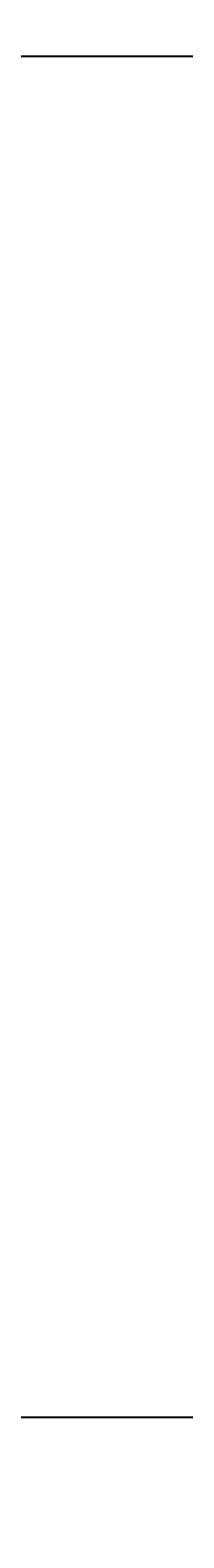
# Model space of a CAD drawing. Units: inches. Extents: x 35362 to 73946, y 43607 to 67532.
# Tile 45 of 134: x 48389 to 48437, y 46091 to 46564. Entities that reach past the tile are written whole.
import ezdxf

# ---------------------------------------------------------------- set-up
doc = ezdxf.new("R2010")
doc.units = ezdxf.units.IN
doc.header["$MEASUREMENT"] = 0
doc.layers.add('A-ANNO-DIMS', color=2, linetype='Continuous', lineweight=18)
doc.styles.get("Standard").update_dxf_attribs({"font": 'arial.ttf'})
doc.dimstyles.get("Standard").update_dxf_attribs({"dimtxt": 0.18, "dimasz": 0.18, "dimexe": 0.18, "dimexo": 0.0625, "dimgap": 0.09, "dimtad": 0, "dimtih": 1, "dimtoh": 1, "dimdec": 4, "dimzin": 0, "dimdsep": 46, "dimtxsty": 'Standard', "dimcen": 0.09, "dimadec": 0, "dimazin": 0, "dimtfac": 1, "dimtdec": 4, "dimtofl": 0, "dimtmove": 0, "dimatfit": 3, "dimfxl": 1, "dimtolj": 1, "dimtzin": 0, "dimarcsym": 0})

# ---------------------------------------------------------------- blocks, each defined once
blk = doc.blocks.new('*D5')
at = {"layer": 'A-ANNO-DIMS', "color": 0, "lineweight": -2, "transparency": 16777216}
for p, q in [((37121.95, 46919.32), (37121.95, 43606.68)), ((69871.5, 45449.83), (69871.5, 43606.68)), ((37122.13, 43606.86), (53496.29, 43606.86)), ((69871.32, 43606.86), (53497.15, 43606.86))]:
    blk.add_line(p, q, dxfattribs=at)
at = {"layer": 'A-ANNO-DIMS', "color": 0, "transparency": 16777216}
for points in [[(37122.13, 43606.89), (37122.13, 43606.83), (37121.95, 43606.86)], [(69871.32, 43606.89), (69871.32, 43606.83), (69871.5, 43606.86)]]:
    blk.add_solid(points, dxfattribs=at)
at = {"layer": 'Defpoints', "color": 0, "transparency": 16777216}
for p in [(37121.95, 46919.38), (69871.5, 45449.89), (69871.5, 43606.86)]:
    blk.add_point(p, dxfattribs=at)
at = {"layer": 'A-ANNO-DIMS', "color": 0, "transparency": 16777216, "insert": (53496.72, 43606.86), "char_height": 0.18, "attachment_point": 5}
blk.add_mtext('\\A1;32750', dxfattribs=at)
blk = doc.blocks.new('*D11')
at = {"layer": 'A-ANNO-DIMS', "color": 0, "lineweight": -2, "transparency": 16777216}
for p, q in [((47978.66, 56028.77), (47978.66, 43606.68)), ((53109.76, 56028.77), (53109.76, 43606.68)), ((47978.84, 43606.86), (50543.87, 43606.86)), ((53109.58, 43606.86), (50544.55, 43606.86))]:
    blk.add_line(p, q, dxfattribs=at)
at = {"layer": 'A-ANNO-DIMS', "color": 0, "transparency": 16777216}
for points in [[(47978.84, 43606.89), (47978.84, 43606.83), (47978.66, 43606.86)], [(53109.58, 43606.89), (53109.58, 43606.83), (53109.76, 43606.86)]]:
    blk.add_solid(points, dxfattribs=at)
at = {"layer": 'Defpoints', "color": 0, "transparency": 16777216}
for p in [(47978.66, 56028.84), (53109.76, 56028.84), (53109.76, 43606.86)]:
    blk.add_point(p, dxfattribs=at)
at = {"layer": 'A-ANNO-DIMS', "color": 0, "transparency": 16777216, "insert": (50544.21, 43606.86), "char_height": 0.18, "attachment_point": 5}
blk.add_mtext('\\A1;5131', dxfattribs=at)
blk = doc.blocks.new('*D13')
at = {"layer": 'A-ANNO-DIMS', "color": 0, "lineweight": -2, "transparency": 16777216}
for p, q in [((48373.49, 51694.02), (48373.49, 43606.68)), ((51029.04, 51694.02), (51029.04, 43606.68)), ((48373.67, 43606.86), (49700.8, 43606.86)), ((51028.86, 43606.86), (49701.73, 43606.86))]:
    blk.add_line(p, q, dxfattribs=at)
at = {"layer": 'A-ANNO-DIMS', "color": 0, "transparency": 16777216}
for points in [[(48373.67, 43606.89), (48373.67, 43606.83), (48373.49, 43606.86)], [(51028.86, 43606.89), (51028.86, 43606.83), (51029.04, 43606.86)]]:
    blk.add_solid(points, dxfattribs=at)
at = {"layer": 'Defpoints', "color": 0, "transparency": 16777216}
for p in [(48373.49, 51694.09), (51029.04, 51694.09), (51029.04, 43606.86)]:
    blk.add_point(p, dxfattribs=at)
at = {"layer": 'A-ANNO-DIMS', "color": 0, "transparency": 16777216, "insert": (49701.27, 43606.86), "char_height": 0.18, "attachment_point": 5}
blk.add_mtext('\\A1;2655.6', dxfattribs=at)
blk = doc.blocks.new('*D67')
at = {"layer": 'A-ANNO-DIMS', "color": 0, "lineweight": -2, "transparency": 16777216}
for p, q in [((56873.54, 53351.53), (35361.77, 53351.53)), ((35361.95, 53351.35), (35361.95, 49400.89)), ((35361.95, 45450.07), (35361.95, 49400.53)), ((53793.58, 45449.89), (35361.77, 45449.89))]:
    blk.add_line(p, q, dxfattribs=at)
at = {"layer": 'A-ANNO-DIMS', "color": 0, "transparency": 16777216}
for points in [[(35361.92, 53351.35), (35361.98, 53351.35), (35361.95, 53351.53)], [(35361.92, 45450.07), (35361.98, 45450.07), (35361.95, 45449.89)]]:
    blk.add_solid(points, dxfattribs=at)
at = {"layer": 'Defpoints', "color": 0, "transparency": 16777216}
for p in [(35361.95, 53351.53), (56873.6, 53351.53), (53793.64, 45449.89)]:
    blk.add_point(p, dxfattribs=at)
at = {"layer": 'A-ANNO-DIMS', "color": 0, "transparency": 16777216, "insert": (35361.95, 49400.71), "char_height": 0.18, "attachment_point": 5}
blk.add_mtext('\\A1;7901.6', dxfattribs=at)
blk = doc.blocks.new('*D76')
at = {"layer": 'A-ANNO-DIMS', "color": 0, "lineweight": -2, "transparency": 16777216}
for p, q in [((54052.84, 46555.29), (35361.77, 46555.29)), ((35361.95, 46555.11), (35361.95, 46342.27)), ((35361.95, 46129.06), (35361.95, 46341.9)), ((53793.58, 46128.88), (35361.77, 46128.88))]:
    blk.add_line(p, q, dxfattribs=at)
at = {"layer": 'A-ANNO-DIMS', "color": 0, "transparency": 16777216}
for points in [[(35361.92, 46555.11), (35361.98, 46555.11), (35361.95, 46555.29)], [(35361.92, 46129.06), (35361.98, 46129.06), (35361.95, 46128.88)]]:
    blk.add_solid(points, dxfattribs=at)
at = {"layer": 'Defpoints', "color": 0, "transparency": 16777216}
for p in [(35361.95, 46555.29), (54052.9, 46555.29), (53793.64, 46128.88)]:
    blk.add_point(p, dxfattribs=at)
at = {"layer": 'A-ANNO-DIMS', "color": 0, "transparency": 16777216, "insert": (35361.95, 46342.09), "char_height": 0.18, "attachment_point": 5}
blk.add_mtext('\\A1;426.4', dxfattribs=at)
blk = doc.blocks.new('*D90')
at = {"layer": 'A-ANNO-DIMS', "color": 0, "lineweight": -2, "transparency": 16777216}
for p, q in [((53707.72, 47291.29), (35361.77, 47291.29)), ((35361.95, 47291.11), (35361.95, 46710.26)), ((35361.95, 46129.06), (35361.95, 46709.9)), ((53793.58, 46128.88), (35361.77, 46128.88))]:
    blk.add_line(p, q, dxfattribs=at)
at = {"layer": 'A-ANNO-DIMS', "color": 0, "transparency": 16777216}
for points in [[(35361.92, 47291.11), (35361.98, 47291.11), (35361.95, 47291.29)], [(35361.92, 46129.06), (35361.98, 46129.06), (35361.95, 46128.88)]]:
    blk.add_solid(points, dxfattribs=at)
at = {"layer": 'Defpoints', "color": 0, "transparency": 16777216}
for p in [(53707.78, 47291.29), (35361.95, 46128.88), (53793.64, 46128.88)]:
    blk.add_point(p, dxfattribs=at)
at = {"layer": 'A-ANNO-DIMS', "color": 0, "transparency": 16777216, "insert": (35361.95, 46710.08), "char_height": 0.18, "attachment_point": 5}
blk.add_mtext('\\A1;1162.4', dxfattribs=at)

msp = doc.modelspace()

# ---------------------------------------------------------------- dimensions: what is measured, and where the dimension line sits
at = {"layer": 'A-ANNO-DIMS'}
for base, p1, p2, override, picture, middle in [((53109.76, 43606.859), (47978.665, 56028.836), (53109.76, 56028.836), {"dimdec": 0, "dimlfac": 1, "dimrnd": 0, "dimzin": 0, "dimdsep": 46, "dimlunit": 2}, '*D11', (50544.212, 43606.859)), ((51029.043, 43606.859), (48373.492, 51694.087), (51029.043, 51694.087), {"dimdec": 1, "dimlfac": 1, "dimrnd": 0, "dimzin": 0, "dimdsep": 46, "dimlunit": 2}, '*D13', (49701.267, 43606.859)), ((69871.496, 43606.859), (37121.949, 46919.381), (69871.496, 45449.894), {"dimdec": 0, "dimlfac": 1, "dimrnd": 0, "dimzin": 0, "dimdsep": 46, "dimlunit": 2}, '*D5', (53496.723, 43606.859))]:
    dim = msp.add_linear_dim(base=base, p1=p1, p2=p2, dimstyle='Standard', override=override, dxfattribs=at)
    dim.commit()
    dim.dimension.update_dxf_attribs({"geometry": picture, "text_midpoint": middle})
for base, p1, p2, picture, middle in [((35361.949, 53351.529), (53793.638, 45449.894), (56873.602, 53351.529), '*D67', (35361.949, 49400.712)), ((35361.949, 46128.878), (53707.781, 47291.285), (53793.638, 46128.878), '*D90', (35361.949, 46710.081)), ((35361.949, 46555.293), (53793.638, 46128.878), (54052.899, 46555.293), '*D76', (35361.949, 46342.086))]:
    dim = msp.add_linear_dim(base=base, p1=p1, p2=p2, angle=90, dimstyle='Standard', override={"dimdec": 1, "dimlfac": 1, "dimrnd": 0, "dimzin": 0, "dimdsep": 46, "dimlunit": 2}, dxfattribs=at)
    dim.commit()
    dim.dimension.update_dxf_attribs({"geometry": picture, "text_midpoint": middle})

doc.saveas('drawing.dxf')
